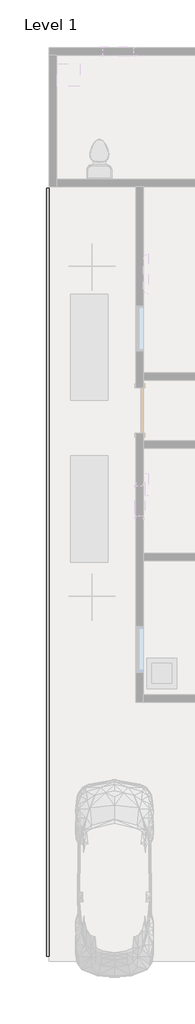
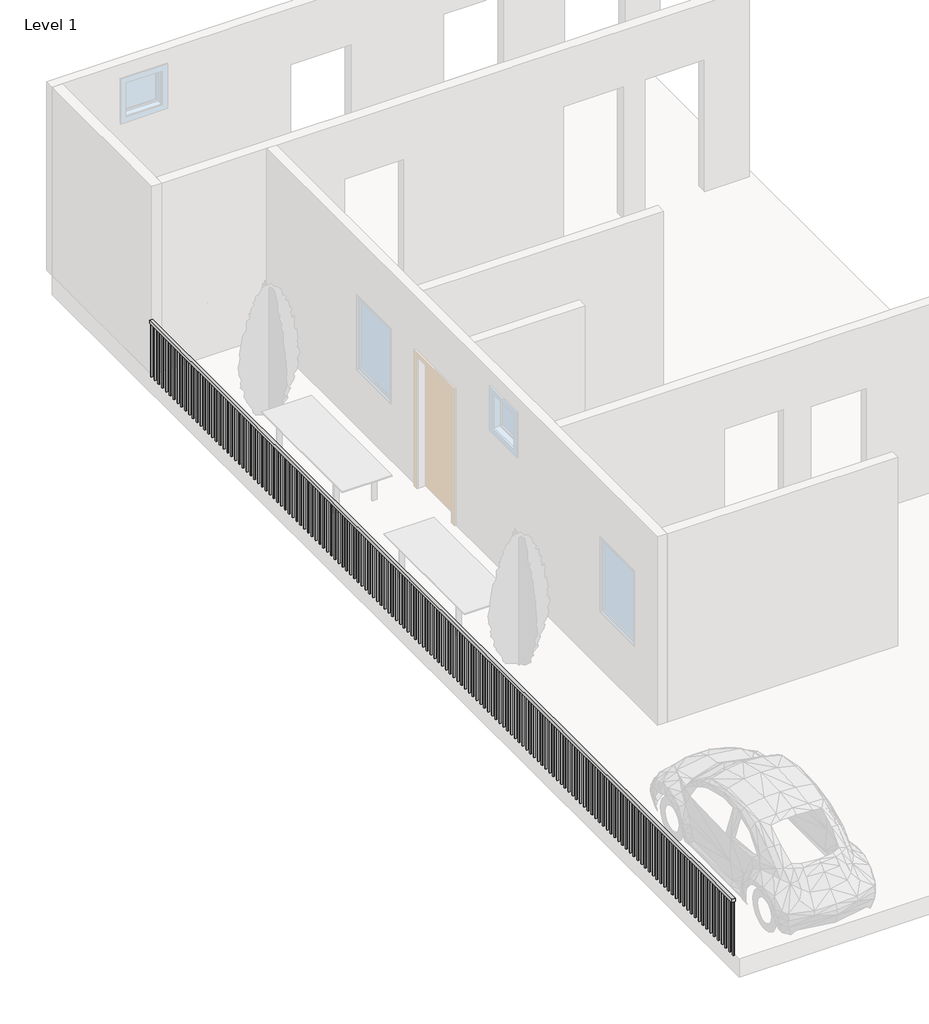
# One storey, part 3 of 4: 1 railing.
"""IFC4 building model written with IfcOpenShell, lengths in millimetres."""

from ifc_helpers import new_model, si_unit, frame, origin, origin_with_axes, place, context, project, spatial, polyline, outline, extrude, element, save

model = new_model("IFC4")

# Units and contexts
model_context = context("Model", 3, world=origin())
ifc_project = project(units=[si_unit("LENGTHUNIT", "METRE", prefix="MILLI")], contexts=[model_context])

# Site, building, storey
site = spatial("IfcSite", under=ifc_project)
building = spatial("IfcBuilding", under=site)
storey = spatial("IfcBuildingStorey", under=building, Name="Level 1", Elevation=0.0)

# Railing
placement = place(None, origin())
element("IfcRailing", 1, ObjectType="Handrail - Rectangular", at=placement, inside=storey, context=model_context, shape_type="SweptSolid", body=[
    extrude(outline(polyline([(-12085.860887, 10860.7910469), (-12035.060887, 10860.7910469), (-12035.060887, -4582.4089531), (-12085.860887, -4582.4089531), (-12085.860887, 10860.7910469)])), frame((0.0, 0.0, 863.6), z_axis=(0.0, 0.0, 1.0), x_axis=(1.0, 0.0, 0.0)), (0.0, 0.0, 1.0), 50.8),
    extrude(outline(polyline([(-12069.985887, -4471.2839531), (-12050.935887, -4471.2839531), (-12050.935887, -4490.3339531), (-12069.985887, -4490.3339531), (-12069.985887, -4471.2839531)])), origin_with_axes(), (0.0, 0.0, 1.0), 863.6),
    extrude(outline(polyline([(-12069.985887, -4369.6839531), (-12050.935887, -4369.6839531), (-12050.935887, -4388.7339531), (-12069.985887, -4388.7339531), (-12069.985887, -4369.6839531)])), origin_with_axes(), (0.0, 0.0, 1.0), 863.6),
    extrude(outline(polyline([(-12069.985887, -4268.0839531), (-12050.935887, -4268.0839531), (-12050.935887, -4287.1339531), (-12069.985887, -4287.1339531), (-12069.985887, -4268.0839531)])), origin_with_axes(), (0.0, 0.0, 1.0), 863.6),
    extrude(outline(polyline([(-12069.985887, -4166.4839531), (-12050.935887, -4166.4839531), (-12050.935887, -4185.5339531), (-12069.985887, -4185.5339531), (-12069.985887, -4166.4839531)])), origin_with_axes(), (0.0, 0.0, 1.0), 863.6),
    extrude(outline(polyline([(-12069.985887, -4064.8839531), (-12050.935887, -4064.8839531), (-12050.935887, -4083.9339531), (-12069.985887, -4083.9339531), (-12069.985887, -4064.8839531)])), origin_with_axes(), (0.0, 0.0, 1.0), 863.6),
    extrude(outline(polyline([(-12069.985887, -3963.2839531), (-12050.935887, -3963.2839531), (-12050.935887, -3982.3339531), (-12069.985887, -3982.3339531), (-12069.985887, -3963.2839531)])), origin_with_axes(), (0.0, 0.0, 1.0), 863.6),
    extrude(outline(polyline([(-12069.985887, -3861.6839531), (-12050.935887, -3861.6839531), (-12050.935887, -3880.7339531), (-12069.985887, -3880.7339531), (-12069.985887, -3861.6839531)])), origin_with_axes(), (0.0, 0.0, 1.0), 863.6),
    extrude(outline(polyline([(-12069.985887, -3760.0839531), (-12050.935887, -3760.0839531), (-12050.935887, -3779.1339531), (-12069.985887, -3779.1339531), (-12069.985887, -3760.0839531)])), origin_with_axes(), (0.0, 0.0, 1.0), 863.6),
    extrude(outline(polyline([(-12069.985887, -3658.4839531), (-12050.935887, -3658.4839531), (-12050.935887, -3677.5339531), (-12069.985887, -3677.5339531), (-12069.985887, -3658.4839531)])), origin_with_axes(), (0.0, 0.0, 1.0), 863.6),
    extrude(outline(polyline([(-12069.985887, -3556.8839531), (-12050.935887, -3556.8839531), (-12050.935887, -3575.9339531), (-12069.985887, -3575.9339531), (-12069.985887, -3556.8839531)])), origin_with_axes(), (0.0, 0.0, 1.0), 863.6),
    extrude(outline(polyline([(-12069.985887, -3455.2839531), (-12050.935887, -3455.2839531), (-12050.935887, -3474.3339531), (-12069.985887, -3474.3339531), (-12069.985887, -3455.2839531)])), origin_with_axes(), (0.0, 0.0, 1.0), 863.6),
    extrude(outline(polyline([(-12069.985887, -3353.6839531), (-12050.935887, -3353.6839531), (-12050.935887, -3372.7339531), (-12069.985887, -3372.7339531), (-12069.985887, -3353.6839531)])), origin_with_axes(), (0.0, 0.0, 1.0), 863.6),
    extrude(outline(polyline([(-12069.985887, -3252.0839531), (-12050.935887, -3252.0839531), (-12050.935887, -3271.1339531), (-12069.985887, -3271.1339531), (-12069.985887, -3252.0839531)])), origin_with_axes(), (0.0, 0.0, 1.0), 863.6),
    extrude(outline(polyline([(-12069.985887, -3150.4839531), (-12050.935887, -3150.4839531), (-12050.935887, -3169.5339531), (-12069.985887, -3169.5339531), (-12069.985887, -3150.4839531)])), origin_with_axes(), (0.0, 0.0, 1.0), 863.6),
    extrude(outline(polyline([(-12069.985887, -3048.8839531), (-12050.935887, -3048.8839531), (-12050.935887, -3067.9339531), (-12069.985887, -3067.9339531), (-12069.985887, -3048.8839531)])), origin_with_axes(), (0.0, 0.0, 1.0), 863.6),
    extrude(outline(polyline([(-12069.985887, -2947.2839531), (-12050.935887, -2947.2839531), (-12050.935887, -2966.3339531), (-12069.985887, -2966.3339531), (-12069.985887, -2947.2839531)])), origin_with_axes(), (0.0, 0.0, 1.0), 863.6),
    extrude(outline(polyline([(-12069.985887, -2845.6839531), (-12050.935887, -2845.6839531), (-12050.935887, -2864.7339531), (-12069.985887, -2864.7339531), (-12069.985887, -2845.6839531)])), origin_with_axes(), (0.0, 0.0, 1.0), 863.6),
    extrude(outline(polyline([(-12069.985887, -2744.0839531), (-12050.935887, -2744.0839531), (-12050.935887, -2763.1339531), (-12069.985887, -2763.1339531), (-12069.985887, -2744.0839531)])), origin_with_axes(), (0.0, 0.0, 1.0), 863.6),
    extrude(outline(polyline([(-12069.985887, -2642.4839531), (-12050.935887, -2642.4839531), (-12050.935887, -2661.5339531), (-12069.985887, -2661.5339531), (-12069.985887, -2642.4839531)])), origin_with_axes(), (0.0, 0.0, 1.0), 863.6),
    extrude(outline(polyline([(-12069.985887, -2540.8839531), (-12050.935887, -2540.8839531), (-12050.935887, -2559.9339531), (-12069.985887, -2559.9339531), (-12069.985887, -2540.8839531)])), origin_with_axes(), (0.0, 0.0, 1.0), 863.6),
    extrude(outline(polyline([(-12069.985887, -2439.2839531), (-12050.935887, -2439.2839531), (-12050.935887, -2458.3339531), (-12069.985887, -2458.3339531), (-12069.985887, -2439.2839531)])), origin_with_axes(), (0.0, 0.0, 1.0), 863.6),
    extrude(outline(polyline([(-12069.985887, -2337.6839531), (-12050.935887, -2337.6839531), (-12050.935887, -2356.7339531), (-12069.985887, -2356.7339531), (-12069.985887, -2337.6839531)])), origin_with_axes(), (0.0, 0.0, 1.0), 863.6),
    extrude(outline(polyline([(-12069.985887, -2236.0839531), (-12050.935887, -2236.0839531), (-12050.935887, -2255.1339531), (-12069.985887, -2255.1339531), (-12069.985887, -2236.0839531)])), origin_with_axes(), (0.0, 0.0, 1.0), 863.6),
    extrude(outline(polyline([(-12069.985887, -2134.4839531), (-12050.935887, -2134.4839531), (-12050.935887, -2153.5339531), (-12069.985887, -2153.5339531), (-12069.985887, -2134.4839531)])), origin_with_axes(), (0.0, 0.0, 1.0), 863.6),
    extrude(outline(polyline([(-12069.985887, -2032.8839531), (-12050.935887, -2032.8839531), (-12050.935887, -2051.9339531), (-12069.985887, -2051.9339531), (-12069.985887, -2032.8839531)])), origin_with_axes(), (0.0, 0.0, 1.0), 863.6),
    extrude(outline(polyline([(-12069.985887, -1931.2839531), (-12050.935887, -1931.2839531), (-12050.935887, -1950.3339531), (-12069.985887, -1950.3339531), (-12069.985887, -1931.2839531)])), origin_with_axes(), (0.0, 0.0, 1.0), 863.6),
    extrude(outline(polyline([(-12069.985887, -1829.6839531), (-12050.935887, -1829.6839531), (-12050.935887, -1848.7339531), (-12069.985887, -1848.7339531), (-12069.985887, -1829.6839531)])), origin_with_axes(), (0.0, 0.0, 1.0), 863.6),
    extrude(outline(polyline([(-12069.985887, -1728.0839531), (-12050.935887, -1728.0839531), (-12050.935887, -1747.1339531), (-12069.985887, -1747.1339531), (-12069.985887, -1728.0839531)])), origin_with_axes(), (0.0, 0.0, 1.0), 863.6),
    extrude(outline(polyline([(-12069.985887, -1626.4839531), (-12050.935887, -1626.4839531), (-12050.935887, -1645.5339531), (-12069.985887, -1645.5339531), (-12069.985887, -1626.4839531)])), origin_with_axes(), (0.0, 0.0, 1.0), 863.6),
    extrude(outline(polyline([(-12069.985887, -1524.8839531), (-12050.935887, -1524.8839531), (-12050.935887, -1543.9339531), (-12069.985887, -1543.9339531), (-12069.985887, -1524.8839531)])), origin_with_axes(), (0.0, 0.0, 1.0), 863.6),
    extrude(outline(polyline([(-12069.985887, -1423.2839531), (-12050.935887, -1423.2839531), (-12050.935887, -1442.3339531), (-12069.985887, -1442.3339531), (-12069.985887, -1423.2839531)])), origin_with_axes(), (0.0, 0.0, 1.0), 863.6),
    extrude(outline(polyline([(-12069.985887, -1321.6839531), (-12050.935887, -1321.6839531), (-12050.935887, -1340.7339531), (-12069.985887, -1340.7339531), (-12069.985887, -1321.6839531)])), origin_with_axes(), (0.0, 0.0, 1.0), 863.6),
    extrude(outline(polyline([(-12069.985887, -1220.0839531), (-12050.935887, -1220.0839531), (-12050.935887, -1239.1339531), (-12069.985887, -1239.1339531), (-12069.985887, -1220.0839531)])), origin_with_axes(), (0.0, 0.0, 1.0), 863.6),
    extrude(outline(polyline([(-12069.985887, -1118.4839531), (-12050.935887, -1118.4839531), (-12050.935887, -1137.5339531), (-12069.985887, -1137.5339531), (-12069.985887, -1118.4839531)])), origin_with_axes(), (0.0, 0.0, 1.0), 863.6),
    extrude(outline(polyline([(-12069.985887, -1016.8839531), (-12050.935887, -1016.8839531), (-12050.935887, -1035.9339531), (-12069.985887, -1035.9339531), (-12069.985887, -1016.8839531)])), origin_with_axes(), (0.0, 0.0, 1.0), 863.6),
    extrude(outline(polyline([(-12069.985887, -915.2839531), (-12050.935887, -915.2839531), (-12050.935887, -934.3339531), (-12069.985887, -934.3339531), (-12069.985887, -915.2839531)])), origin_with_axes(), (0.0, 0.0, 1.0), 863.6),
    extrude(outline(polyline([(-12069.985887, -813.6839531), (-12050.935887, -813.6839531), (-12050.935887, -832.7339531), (-12069.985887, -832.7339531), (-12069.985887, -813.6839531)])), origin_with_axes(), (0.0, 0.0, 1.0), 863.6),
    extrude(outline(polyline([(-12069.985887, -712.0839531), (-12050.935887, -712.0839531), (-12050.935887, -731.1339531), (-12069.985887, -731.1339531), (-12069.985887, -712.0839531)])), origin_with_axes(), (0.0, 0.0, 1.0), 863.6),
    extrude(outline(polyline([(-12069.985887, -610.4839531), (-12050.935887, -610.4839531), (-12050.935887, -629.5339531), (-12069.985887, -629.5339531), (-12069.985887, -610.4839531)])), origin_with_axes(), (0.0, 0.0, 1.0), 863.6),
    extrude(outline(polyline([(-12069.985887, -508.8839531), (-12050.935887, -508.8839531), (-12050.935887, -527.9339531), (-12069.985887, -527.9339531), (-12069.985887, -508.8839531)])), origin_with_axes(), (0.0, 0.0, 1.0), 863.6),
    extrude(outline(polyline([(-12069.985887, -407.2839531), (-12050.935887, -407.2839531), (-12050.935887, -426.3339531), (-12069.985887, -426.3339531), (-12069.985887, -407.2839531)])), origin_with_axes(), (0.0, 0.0, 1.0), 863.6),
    extrude(outline(polyline([(-12069.985887, -305.6839531), (-12050.935887, -305.6839531), (-12050.935887, -324.7339531), (-12069.985887, -324.7339531), (-12069.985887, -305.6839531)])), origin_with_axes(), (0.0, 0.0, 1.0), 863.6),
    extrude(outline(polyline([(-12069.985887, -204.0839531), (-12050.935887, -204.0839531), (-12050.935887, -223.1339531), (-12069.985887, -223.1339531), (-12069.985887, -204.0839531)])), origin_with_axes(), (0.0, 0.0, 1.0), 863.6),
    extrude(outline(polyline([(-12069.985887, -102.4839531), (-12050.935887, -102.4839531), (-12050.935887, -121.5339531), (-12069.985887, -121.5339531), (-12069.985887, -102.4839531)])), origin_with_axes(), (0.0, 0.0, 1.0), 863.6),
    extrude(outline(polyline([(-12069.985887, -0.8839531), (-12050.935887, -0.8839531), (-12050.935887, -19.9339531), (-12069.985887, -19.9339531), (-12069.985887, -0.8839531)])), origin_with_axes(), (0.0, 0.0, 1.0), 863.6),
    extrude(outline(polyline([(-12069.985887, 100.7160469), (-12050.935887, 100.7160469), (-12050.935887, 81.6660469), (-12069.985887, 81.6660469), (-12069.985887, 100.7160469)])), origin_with_axes(), (0.0, 0.0, 1.0), 863.6),
    extrude(outline(polyline([(-12069.985887, 202.3160469), (-12050.935887, 202.3160469), (-12050.935887, 183.2660469), (-12069.985887, 183.2660469), (-12069.985887, 202.3160469)])), origin_with_axes(), (0.0, 0.0, 1.0), 863.6),
    extrude(outline(polyline([(-12069.985887, 303.9160469), (-12050.935887, 303.9160469), (-12050.935887, 284.8660469), (-12069.985887, 284.8660469), (-12069.985887, 303.9160469)])), origin_with_axes(), (0.0, 0.0, 1.0), 863.6),
    extrude(outline(polyline([(-12069.985887, 405.5160469), (-12050.935887, 405.5160469), (-12050.935887, 386.4660469), (-12069.985887, 386.4660469), (-12069.985887, 405.5160469)])), origin_with_axes(), (0.0, 0.0, 1.0), 863.6),
    extrude(outline(polyline([(-12069.985887, 507.1160469), (-12050.935887, 507.1160469), (-12050.935887, 488.0660469), (-12069.985887, 488.0660469), (-12069.985887, 507.1160469)])), origin_with_axes(), (0.0, 0.0, 1.0), 863.6),
    extrude(outline(polyline([(-12069.985887, 608.7160469), (-12050.935887, 608.7160469), (-12050.935887, 589.6660469), (-12069.985887, 589.6660469), (-12069.985887, 608.7160469)])), origin_with_axes(), (0.0, 0.0, 1.0), 863.6),
    extrude(outline(polyline([(-12069.985887, 710.3160469), (-12050.935887, 710.3160469), (-12050.935887, 691.2660469), (-12069.985887, 691.2660469), (-12069.985887, 710.3160469)])), origin_with_axes(), (0.0, 0.0, 1.0), 863.6),
    extrude(outline(polyline([(-12069.985887, 811.9160469), (-12050.935887, 811.9160469), (-12050.935887, 792.8660469), (-12069.985887, 792.8660469), (-12069.985887, 811.9160469)])), origin_with_axes(), (0.0, 0.0, 1.0), 863.6),
    extrude(outline(polyline([(-12069.985887, 913.5160469), (-12050.935887, 913.5160469), (-12050.935887, 894.4660469), (-12069.985887, 894.4660469), (-12069.985887, 913.5160469)])), origin_with_axes(), (0.0, 0.0, 1.0), 863.6),
    extrude(outline(polyline([(-12069.985887, 1015.1160469), (-12050.935887, 1015.1160469), (-12050.935887, 996.0660469), (-12069.985887, 996.0660469), (-12069.985887, 1015.1160469)])), origin_with_axes(), (0.0, 0.0, 1.0), 863.6),
    extrude(outline(polyline([(-12069.985887, 1116.7160469), (-12050.935887, 1116.7160469), (-12050.935887, 1097.6660469), (-12069.985887, 1097.6660469), (-12069.985887, 1116.7160469)])), origin_with_axes(), (0.0, 0.0, 1.0), 863.6),
    extrude(outline(polyline([(-12069.985887, 1218.3160469), (-12050.935887, 1218.3160469), (-12050.935887, 1199.2660469), (-12069.985887, 1199.2660469), (-12069.985887, 1218.3160469)])), origin_with_axes(), (0.0, 0.0, 1.0), 863.6),
    extrude(outline(polyline([(-12069.985887, 1319.9160469), (-12050.935887, 1319.9160469), (-12050.935887, 1300.8660469), (-12069.985887, 1300.8660469), (-12069.985887, 1319.9160469)])), origin_with_axes(), (0.0, 0.0, 1.0), 863.6),
    extrude(outline(polyline([(-12069.985887, 1421.5160469), (-12050.935887, 1421.5160469), (-12050.935887, 1402.4660469), (-12069.985887, 1402.4660469), (-12069.985887, 1421.5160469)])), origin_with_axes(), (0.0, 0.0, 1.0), 863.6),
    extrude(outline(polyline([(-12069.985887, 1523.1160469), (-12050.935887, 1523.1160469), (-12050.935887, 1504.0660469), (-12069.985887, 1504.0660469), (-12069.985887, 1523.1160469)])), origin_with_axes(), (0.0, 0.0, 1.0), 863.6),
    extrude(outline(polyline([(-12069.985887, 1624.7160469), (-12050.935887, 1624.7160469), (-12050.935887, 1605.6660469), (-12069.985887, 1605.6660469), (-12069.985887, 1624.7160469)])), origin_with_axes(), (0.0, 0.0, 1.0), 863.6),
    extrude(outline(polyline([(-12069.985887, 1726.3160469), (-12050.935887, 1726.3160469), (-12050.935887, 1707.2660469), (-12069.985887, 1707.2660469), (-12069.985887, 1726.3160469)])), origin_with_axes(), (0.0, 0.0, 1.0), 863.6),
    extrude(outline(polyline([(-12069.985887, 1827.9160469), (-12050.935887, 1827.9160469), (-12050.935887, 1808.8660469), (-12069.985887, 1808.8660469), (-12069.985887, 1827.9160469)])), origin_with_axes(), (0.0, 0.0, 1.0), 863.6),
    extrude(outline(polyline([(-12069.985887, 1929.5160469), (-12050.935887, 1929.5160469), (-12050.935887, 1910.4660469), (-12069.985887, 1910.4660469), (-12069.985887, 1929.5160469)])), origin_with_axes(), (0.0, 0.0, 1.0), 863.6),
    extrude(outline(polyline([(-12069.985887, 2031.1160469), (-12050.935887, 2031.1160469), (-12050.935887, 2012.0660469), (-12069.985887, 2012.0660469), (-12069.985887, 2031.1160469)])), origin_with_axes(), (0.0, 0.0, 1.0), 863.6),
    extrude(outline(polyline([(-12069.985887, 2132.7160469), (-12050.935887, 2132.7160469), (-12050.935887, 2113.6660469), (-12069.985887, 2113.6660469), (-12069.985887, 2132.7160469)])), origin_with_axes(), (0.0, 0.0, 1.0), 863.6),
    extrude(outline(polyline([(-12069.985887, 2234.3160469), (-12050.935887, 2234.3160469), (-12050.935887, 2215.2660469), (-12069.985887, 2215.2660469), (-12069.985887, 2234.3160469)])), origin_with_axes(), (0.0, 0.0, 1.0), 863.6),
    extrude(outline(polyline([(-12069.985887, 2335.9160469), (-12050.935887, 2335.9160469), (-12050.935887, 2316.8660469), (-12069.985887, 2316.8660469), (-12069.985887, 2335.9160469)])), origin_with_axes(), (0.0, 0.0, 1.0), 863.6),
    extrude(outline(polyline([(-12069.985887, 2437.5160469), (-12050.935887, 2437.5160469), (-12050.935887, 2418.4660469), (-12069.985887, 2418.4660469), (-12069.985887, 2437.5160469)])), origin_with_axes(), (0.0, 0.0, 1.0), 863.6),
    extrude(outline(polyline([(-12069.985887, 2539.1160469), (-12050.935887, 2539.1160469), (-12050.935887, 2520.0660469), (-12069.985887, 2520.0660469), (-12069.985887, 2539.1160469)])), origin_with_axes(), (0.0, 0.0, 1.0), 863.6),
    extrude(outline(polyline([(-12069.985887, 2640.7160469), (-12050.935887, 2640.7160469), (-12050.935887, 2621.6660469), (-12069.985887, 2621.6660469), (-12069.985887, 2640.7160469)])), origin_with_axes(), (0.0, 0.0, 1.0), 863.6),
    extrude(outline(polyline([(-12069.985887, 2742.3160469), (-12050.935887, 2742.3160469), (-12050.935887, 2723.2660469), (-12069.985887, 2723.2660469), (-12069.985887, 2742.3160469)])), origin_with_axes(), (0.0, 0.0, 1.0), 863.6),
    extrude(outline(polyline([(-12069.985887, 2843.9160469), (-12050.935887, 2843.9160469), (-12050.935887, 2824.8660469), (-12069.985887, 2824.8660469), (-12069.985887, 2843.9160469)])), origin_with_axes(), (0.0, 0.0, 1.0), 863.6),
    extrude(outline(polyline([(-12069.985887, 2945.5160469), (-12050.935887, 2945.5160469), (-12050.935887, 2926.4660469), (-12069.985887, 2926.4660469), (-12069.985887, 2945.5160469)])), origin_with_axes(), (0.0, 0.0, 1.0), 863.6),
    extrude(outline(polyline([(-12069.985887, 3047.1160469), (-12050.935887, 3047.1160469), (-12050.935887, 3028.0660469), (-12069.985887, 3028.0660469), (-12069.985887, 3047.1160469)])), origin_with_axes(), (0.0, 0.0, 1.0), 863.6),
    extrude(outline(polyline([(-12069.985887, 3148.7160469), (-12050.935887, 3148.7160469), (-12050.935887, 3129.6660469), (-12069.985887, 3129.6660469), (-12069.985887, 3148.7160469)])), origin_with_axes(), (0.0, 0.0, 1.0), 863.6),
    extrude(outline(polyline([(-12069.985887, 3250.3160469), (-12050.935887, 3250.3160469), (-12050.935887, 3231.2660469), (-12069.985887, 3231.2660469), (-12069.985887, 3250.3160469)])), origin_with_axes(), (0.0, 0.0, 1.0), 863.6),
    extrude(outline(polyline([(-12069.985887, 3351.9160469), (-12050.935887, 3351.9160469), (-12050.935887, 3332.8660469), (-12069.985887, 3332.8660469), (-12069.985887, 3351.9160469)])), origin_with_axes(), (0.0, 0.0, 1.0), 863.6),
    extrude(outline(polyline([(-12069.985887, 3453.5160469), (-12050.935887, 3453.5160469), (-12050.935887, 3434.4660469), (-12069.985887, 3434.4660469), (-12069.985887, 3453.5160469)])), origin_with_axes(), (0.0, 0.0, 1.0), 863.6),
    extrude(outline(polyline([(-12069.985887, 3555.1160469), (-12050.935887, 3555.1160469), (-12050.935887, 3536.0660469), (-12069.985887, 3536.0660469), (-12069.985887, 3555.1160469)])), origin_with_axes(), (0.0, 0.0, 1.0), 863.6),
    extrude(outline(polyline([(-12069.985887, 3656.7160469), (-12050.935887, 3656.7160469), (-12050.935887, 3637.6660469), (-12069.985887, 3637.6660469), (-12069.985887, 3656.7160469)])), origin_with_axes(), (0.0, 0.0, 1.0), 863.6),
    extrude(outline(polyline([(-12069.985887, 3758.3160469), (-12050.935887, 3758.3160469), (-12050.935887, 3739.2660469), (-12069.985887, 3739.2660469), (-12069.985887, 3758.3160469)])), origin_with_axes(), (0.0, 0.0, 1.0), 863.6),
    extrude(outline(polyline([(-12069.985887, 3859.9160469), (-12050.935887, 3859.9160469), (-12050.935887, 3840.8660469), (-12069.985887, 3840.8660469), (-12069.985887, 3859.9160469)])), origin_with_axes(), (0.0, 0.0, 1.0), 863.6),
    extrude(outline(polyline([(-12069.985887, 3961.5160469), (-12050.935887, 3961.5160469), (-12050.935887, 3942.4660469), (-12069.985887, 3942.4660469), (-12069.985887, 3961.5160469)])), origin_with_axes(), (0.0, 0.0, 1.0), 863.6),
    extrude(outline(polyline([(-12069.985887, 4063.1160469), (-12050.935887, 4063.1160469), (-12050.935887, 4044.0660469), (-12069.985887, 4044.0660469), (-12069.985887, 4063.1160469)])), origin_with_axes(), (0.0, 0.0, 1.0), 863.6),
    extrude(outline(polyline([(-12069.985887, 4164.7160469), (-12050.935887, 4164.7160469), (-12050.935887, 4145.6660469), (-12069.985887, 4145.6660469), (-12069.985887, 4164.7160469)])), origin_with_axes(), (0.0, 0.0, 1.0), 863.6),
    extrude(outline(polyline([(-12069.985887, 4266.3160469), (-12050.935887, 4266.3160469), (-12050.935887, 4247.2660469), (-12069.985887, 4247.2660469), (-12069.985887, 4266.3160469)])), origin_with_axes(), (0.0, 0.0, 1.0), 863.6),
    extrude(outline(polyline([(-12069.985887, 4367.9160469), (-12050.935887, 4367.9160469), (-12050.935887, 4348.8660469), (-12069.985887, 4348.8660469), (-12069.985887, 4367.9160469)])), origin_with_axes(), (0.0, 0.0, 1.0), 863.6),
    extrude(outline(polyline([(-12069.985887, 4469.5160469), (-12050.935887, 4469.5160469), (-12050.935887, 4450.4660469), (-12069.985887, 4450.4660469), (-12069.985887, 4469.5160469)])), origin_with_axes(), (0.0, 0.0, 1.0), 863.6),
    extrude(outline(polyline([(-12069.985887, 4571.1160469), (-12050.935887, 4571.1160469), (-12050.935887, 4552.0660469), (-12069.985887, 4552.0660469), (-12069.985887, 4571.1160469)])), origin_with_axes(), (0.0, 0.0, 1.0), 863.6),
    extrude(outline(polyline([(-12069.985887, 4672.7160469), (-12050.935887, 4672.7160469), (-12050.935887, 4653.6660469), (-12069.985887, 4653.6660469), (-12069.985887, 4672.7160469)])), origin_with_axes(), (0.0, 0.0, 1.0), 863.6),
    extrude(outline(polyline([(-12069.985887, 4774.3160469), (-12050.935887, 4774.3160469), (-12050.935887, 4755.2660469), (-12069.985887, 4755.2660469), (-12069.985887, 4774.3160469)])), origin_with_axes(), (0.0, 0.0, 1.0), 863.6),
    extrude(outline(polyline([(-12069.985887, 4875.9160469), (-12050.935887, 4875.9160469), (-12050.935887, 4856.8660469), (-12069.985887, 4856.8660469), (-12069.985887, 4875.9160469)])), origin_with_axes(), (0.0, 0.0, 1.0), 863.6),
    extrude(outline(polyline([(-12069.985887, 4977.5160469), (-12050.935887, 4977.5160469), (-12050.935887, 4958.4660469), (-12069.985887, 4958.4660469), (-12069.985887, 4977.5160469)])), origin_with_axes(), (0.0, 0.0, 1.0), 863.6),
    extrude(outline(polyline([(-12069.985887, 5079.1160469), (-12050.935887, 5079.1160469), (-12050.935887, 5060.0660469), (-12069.985887, 5060.0660469), (-12069.985887, 5079.1160469)])), origin_with_axes(), (0.0, 0.0, 1.0), 863.6),
    extrude(outline(polyline([(-12069.985887, 5180.7160469), (-12050.935887, 5180.7160469), (-12050.935887, 5161.6660469), (-12069.985887, 5161.6660469), (-12069.985887, 5180.7160469)])), origin_with_axes(), (0.0, 0.0, 1.0), 863.6),
    extrude(outline(polyline([(-12069.985887, 5282.3160469), (-12050.935887, 5282.3160469), (-12050.935887, 5263.2660469), (-12069.985887, 5263.2660469), (-12069.985887, 5282.3160469)])), origin_with_axes(), (0.0, 0.0, 1.0), 863.6),
    extrude(outline(polyline([(-12069.985887, 5383.9160469), (-12050.935887, 5383.9160469), (-12050.935887, 5364.8660469), (-12069.985887, 5364.8660469), (-12069.985887, 5383.9160469)])), origin_with_axes(), (0.0, 0.0, 1.0), 863.6),
    extrude(outline(polyline([(-12069.985887, 5485.5160469), (-12050.935887, 5485.5160469), (-12050.935887, 5466.4660469), (-12069.985887, 5466.4660469), (-12069.985887, 5485.5160469)])), origin_with_axes(), (0.0, 0.0, 1.0), 863.6),
    extrude(outline(polyline([(-12069.985887, 5587.1160469), (-12050.935887, 5587.1160469), (-12050.935887, 5568.0660469), (-12069.985887, 5568.0660469), (-12069.985887, 5587.1160469)])), origin_with_axes(), (0.0, 0.0, 1.0), 863.6),
    extrude(outline(polyline([(-12069.985887, 5688.7160469), (-12050.935887, 5688.7160469), (-12050.935887, 5669.6660469), (-12069.985887, 5669.6660469), (-12069.985887, 5688.7160469)])), origin_with_axes(), (0.0, 0.0, 1.0), 863.6),
    extrude(outline(polyline([(-12069.985887, 5790.3160469), (-12050.935887, 5790.3160469), (-12050.935887, 5771.2660469), (-12069.985887, 5771.2660469), (-12069.985887, 5790.3160469)])), origin_with_axes(), (0.0, 0.0, 1.0), 863.6),
    extrude(outline(polyline([(-12069.985887, 5891.9160469), (-12050.935887, 5891.9160469), (-12050.935887, 5872.8660469), (-12069.985887, 5872.8660469), (-12069.985887, 5891.9160469)])), origin_with_axes(), (0.0, 0.0, 1.0), 863.6),
    extrude(outline(polyline([(-12069.985887, 5993.5160469), (-12050.935887, 5993.5160469), (-12050.935887, 5974.4660469), (-12069.985887, 5974.4660469), (-12069.985887, 5993.5160469)])), origin_with_axes(), (0.0, 0.0, 1.0), 863.6),
    extrude(outline(polyline([(-12069.985887, 6095.1160469), (-12050.935887, 6095.1160469), (-12050.935887, 6076.0660469), (-12069.985887, 6076.0660469), (-12069.985887, 6095.1160469)])), origin_with_axes(), (0.0, 0.0, 1.0), 863.6),
    extrude(outline(polyline([(-12069.985887, 6196.7160469), (-12050.935887, 6196.7160469), (-12050.935887, 6177.6660469), (-12069.985887, 6177.6660469), (-12069.985887, 6196.7160469)])), origin_with_axes(), (0.0, 0.0, 1.0), 863.6),
    extrude(outline(polyline([(-12069.985887, 6298.3160469), (-12050.935887, 6298.3160469), (-12050.935887, 6279.2660469), (-12069.985887, 6279.2660469), (-12069.985887, 6298.3160469)])), origin_with_axes(), (0.0, 0.0, 1.0), 863.6),
    extrude(outline(polyline([(-12069.985887, 6399.9160469), (-12050.935887, 6399.9160469), (-12050.935887, 6380.8660469), (-12069.985887, 6380.8660469), (-12069.985887, 6399.9160469)])), origin_with_axes(), (0.0, 0.0, 1.0), 863.6),
    extrude(outline(polyline([(-12069.985887, 6501.5160469), (-12050.935887, 6501.5160469), (-12050.935887, 6482.4660469), (-12069.985887, 6482.4660469), (-12069.985887, 6501.5160469)])), origin_with_axes(), (0.0, 0.0, 1.0), 863.6),
    extrude(outline(polyline([(-12069.985887, 6603.1160469), (-12050.935887, 6603.1160469), (-12050.935887, 6584.0660469), (-12069.985887, 6584.0660469), (-12069.985887, 6603.1160469)])), origin_with_axes(), (0.0, 0.0, 1.0), 863.6),
    extrude(outline(polyline([(-12069.985887, 6704.7160469), (-12050.935887, 6704.7160469), (-12050.935887, 6685.6660469), (-12069.985887, 6685.6660469), (-12069.985887, 6704.7160469)])), origin_with_axes(), (0.0, 0.0, 1.0), 863.6),
    extrude(outline(polyline([(-12069.985887, 6806.3160469), (-12050.935887, 6806.3160469), (-12050.935887, 6787.2660469), (-12069.985887, 6787.2660469), (-12069.985887, 6806.3160469)])), origin_with_axes(), (0.0, 0.0, 1.0), 863.6),
    extrude(outline(polyline([(-12069.985887, 6907.9160469), (-12050.935887, 6907.9160469), (-12050.935887, 6888.8660469), (-12069.985887, 6888.8660469), (-12069.985887, 6907.9160469)])), origin_with_axes(), (0.0, 0.0, 1.0), 863.6),
    extrude(outline(polyline([(-12069.985887, 7009.5160469), (-12050.935887, 7009.5160469), (-12050.935887, 6990.4660469), (-12069.985887, 6990.4660469), (-12069.985887, 7009.5160469)])), origin_with_axes(), (0.0, 0.0, 1.0), 863.6),
    extrude(outline(polyline([(-12069.985887, 7111.1160469), (-12050.935887, 7111.1160469), (-12050.935887, 7092.0660469), (-12069.985887, 7092.0660469), (-12069.985887, 7111.1160469)])), origin_with_axes(), (0.0, 0.0, 1.0), 863.6),
    extrude(outline(polyline([(-12069.985887, 7212.7160469), (-12050.935887, 7212.7160469), (-12050.935887, 7193.6660469), (-12069.985887, 7193.6660469), (-12069.985887, 7212.7160469)])), origin_with_axes(), (0.0, 0.0, 1.0), 863.6),
    extrude(outline(polyline([(-12069.985887, 7314.3160469), (-12050.935887, 7314.3160469), (-12050.935887, 7295.2660469), (-12069.985887, 7295.2660469), (-12069.985887, 7314.3160469)])), origin_with_axes(), (0.0, 0.0, 1.0), 863.6),
    extrude(outline(polyline([(-12069.985887, 7415.9160469), (-12050.935887, 7415.9160469), (-12050.935887, 7396.8660469), (-12069.985887, 7396.8660469), (-12069.985887, 7415.9160469)])), origin_with_axes(), (0.0, 0.0, 1.0), 863.6),
    extrude(outline(polyline([(-12069.985887, 7517.5160469), (-12050.935887, 7517.5160469), (-12050.935887, 7498.4660469), (-12069.985887, 7498.4660469), (-12069.985887, 7517.5160469)])), origin_with_axes(), (0.0, 0.0, 1.0), 863.6),
    extrude(outline(polyline([(-12069.985887, 7619.1160469), (-12050.935887, 7619.1160469), (-12050.935887, 7600.0660469), (-12069.985887, 7600.0660469), (-12069.985887, 7619.1160469)])), origin_with_axes(), (0.0, 0.0, 1.0), 863.6),
    extrude(outline(polyline([(-12069.985887, 7720.7160469), (-12050.935887, 7720.7160469), (-12050.935887, 7701.6660469), (-12069.985887, 7701.6660469), (-12069.985887, 7720.7160469)])), origin_with_axes(), (0.0, 0.0, 1.0), 863.6),
    extrude(outline(polyline([(-12069.985887, 7822.3160469), (-12050.935887, 7822.3160469), (-12050.935887, 7803.2660469), (-12069.985887, 7803.2660469), (-12069.985887, 7822.3160469)])), origin_with_axes(), (0.0, 0.0, 1.0), 863.6),
    extrude(outline(polyline([(-12069.985887, 7923.9160469), (-12050.935887, 7923.9160469), (-12050.935887, 7904.8660469), (-12069.985887, 7904.8660469), (-12069.985887, 7923.9160469)])), origin_with_axes(), (0.0, 0.0, 1.0), 863.6),
    extrude(outline(polyline([(-12069.985887, 8025.5160469), (-12050.935887, 8025.5160469), (-12050.935887, 8006.4660469), (-12069.985887, 8006.4660469), (-12069.985887, 8025.5160469)])), origin_with_axes(), (0.0, 0.0, 1.0), 863.6),
    extrude(outline(polyline([(-12069.985887, 8127.1160469), (-12050.935887, 8127.1160469), (-12050.935887, 8108.0660469), (-12069.985887, 8108.0660469), (-12069.985887, 8127.1160469)])), origin_with_axes(), (0.0, 0.0, 1.0), 863.6),
    extrude(outline(polyline([(-12069.985887, 8228.7160469), (-12050.935887, 8228.7160469), (-12050.935887, 8209.6660469), (-12069.985887, 8209.6660469), (-12069.985887, 8228.7160469)])), origin_with_axes(), (0.0, 0.0, 1.0), 863.6),
    extrude(outline(polyline([(-12069.985887, 8330.3160469), (-12050.935887, 8330.3160469), (-12050.935887, 8311.2660469), (-12069.985887, 8311.2660469), (-12069.985887, 8330.3160469)])), origin_with_axes(), (0.0, 0.0, 1.0), 863.6),
    extrude(outline(polyline([(-12069.985887, 8431.9160469), (-12050.935887, 8431.9160469), (-12050.935887, 8412.8660469), (-12069.985887, 8412.8660469), (-12069.985887, 8431.9160469)])), origin_with_axes(), (0.0, 0.0, 1.0), 863.6),
    extrude(outline(polyline([(-12069.985887, 8533.5160469), (-12050.935887, 8533.5160469), (-12050.935887, 8514.4660469), (-12069.985887, 8514.4660469), (-12069.985887, 8533.5160469)])), origin_with_axes(), (0.0, 0.0, 1.0), 863.6),
    extrude(outline(polyline([(-12069.985887, 8635.1160469), (-12050.935887, 8635.1160469), (-12050.935887, 8616.0660469), (-12069.985887, 8616.0660469), (-12069.985887, 8635.1160469)])), origin_with_axes(), (0.0, 0.0, 1.0), 863.6),
    extrude(outline(polyline([(-12069.985887, 8736.7160469), (-12050.935887, 8736.7160469), (-12050.935887, 8717.6660469), (-12069.985887, 8717.6660469), (-12069.985887, 8736.7160469)])), origin_with_axes(), (0.0, 0.0, 1.0), 863.6),
    extrude(outline(polyline([(-12069.985887, 8838.3160469), (-12050.935887, 8838.3160469), (-12050.935887, 8819.2660469), (-12069.985887, 8819.2660469), (-12069.985887, 8838.3160469)])), origin_with_axes(), (0.0, 0.0, 1.0), 863.6),
    extrude(outline(polyline([(-12069.985887, 8939.9160469), (-12050.935887, 8939.9160469), (-12050.935887, 8920.8660469), (-12069.985887, 8920.8660469), (-12069.985887, 8939.9160469)])), origin_with_axes(), (0.0, 0.0, 1.0), 863.6),
    extrude(outline(polyline([(-12069.985887, 9041.5160469), (-12050.935887, 9041.5160469), (-12050.935887, 9022.4660469), (-12069.985887, 9022.4660469), (-12069.985887, 9041.5160469)])), origin_with_axes(), (0.0, 0.0, 1.0), 863.6),
    extrude(outline(polyline([(-12069.985887, 9143.1160469), (-12050.935887, 9143.1160469), (-12050.935887, 9124.0660469), (-12069.985887, 9124.0660469), (-12069.985887, 9143.1160469)])), origin_with_axes(), (0.0, 0.0, 1.0), 863.6),
    extrude(outline(polyline([(-12069.985887, 9244.7160469), (-12050.935887, 9244.7160469), (-12050.935887, 9225.6660469), (-12069.985887, 9225.6660469), (-12069.985887, 9244.7160469)])), origin_with_axes(), (0.0, 0.0, 1.0), 863.6),
    extrude(outline(polyline([(-12069.985887, 9346.3160469), (-12050.935887, 9346.3160469), (-12050.935887, 9327.2660469), (-12069.985887, 9327.2660469), (-12069.985887, 9346.3160469)])), origin_with_axes(), (0.0, 0.0, 1.0), 863.6),
    extrude(outline(polyline([(-12069.985887, 9447.9160469), (-12050.935887, 9447.9160469), (-12050.935887, 9428.8660469), (-12069.985887, 9428.8660469), (-12069.985887, 9447.9160469)])), origin_with_axes(), (0.0, 0.0, 1.0), 863.6),
    extrude(outline(polyline([(-12069.985887, 9549.5160469), (-12050.935887, 9549.5160469), (-12050.935887, 9530.4660469), (-12069.985887, 9530.4660469), (-12069.985887, 9549.5160469)])), origin_with_axes(), (0.0, 0.0, 1.0), 863.6),
    extrude(outline(polyline([(-12069.985887, 9651.1160469), (-12050.935887, 9651.1160469), (-12050.935887, 9632.0660469), (-12069.985887, 9632.0660469), (-12069.985887, 9651.1160469)])), origin_with_axes(), (0.0, 0.0, 1.0), 863.6),
    extrude(outline(polyline([(-12069.985887, 9752.7160469), (-12050.935887, 9752.7160469), (-12050.935887, 9733.6660469), (-12069.985887, 9733.6660469), (-12069.985887, 9752.7160469)])), origin_with_axes(), (0.0, 0.0, 1.0), 863.6),
    extrude(outline(polyline([(-12069.985887, 9854.3160469), (-12050.935887, 9854.3160469), (-12050.935887, 9835.2660469), (-12069.985887, 9835.2660469), (-12069.985887, 9854.3160469)])), origin_with_axes(), (0.0, 0.0, 1.0), 863.6),
    extrude(outline(polyline([(-12069.985887, 9955.9160469), (-12050.935887, 9955.9160469), (-12050.935887, 9936.8660469), (-12069.985887, 9936.8660469), (-12069.985887, 9955.9160469)])), origin_with_axes(), (0.0, 0.0, 1.0), 863.6),
    extrude(outline(polyline([(-12069.985887, 10057.5160469), (-12050.935887, 10057.5160469), (-12050.935887, 10038.4660469), (-12069.985887, 10038.4660469), (-12069.985887, 10057.5160469)])), origin_with_axes(), (0.0, 0.0, 1.0), 863.6),
    extrude(outline(polyline([(-12069.985887, 10159.1160469), (-12050.935887, 10159.1160469), (-12050.935887, 10140.0660469), (-12069.985887, 10140.0660469), (-12069.985887, 10159.1160469)])), origin_with_axes(), (0.0, 0.0, 1.0), 863.6),
    extrude(outline(polyline([(-12069.985887, 10260.7160469), (-12050.935887, 10260.7160469), (-12050.935887, 10241.6660469), (-12069.985887, 10241.6660469), (-12069.985887, 10260.7160469)])), origin_with_axes(), (0.0, 0.0, 1.0), 863.6),
    extrude(outline(polyline([(-12069.985887, 10362.3160469), (-12050.935887, 10362.3160469), (-12050.935887, 10343.2660469), (-12069.985887, 10343.2660469), (-12069.985887, 10362.3160469)])), origin_with_axes(), (0.0, 0.0, 1.0), 863.6),
    extrude(outline(polyline([(-12069.985887, 10463.9160469), (-12050.935887, 10463.9160469), (-12050.935887, 10444.8660469), (-12069.985887, 10444.8660469), (-12069.985887, 10463.9160469)])), origin_with_axes(), (0.0, 0.0, 1.0), 863.6),
    extrude(outline(polyline([(-12069.985887, 10565.5160469), (-12050.935887, 10565.5160469), (-12050.935887, 10546.4660469), (-12069.985887, 10546.4660469), (-12069.985887, 10565.5160469)])), origin_with_axes(), (0.0, 0.0, 1.0), 863.6),
    extrude(outline(polyline([(-12069.985887, 10667.1160469), (-12050.935887, 10667.1160469), (-12050.935887, 10648.0660469), (-12069.985887, 10648.0660469), (-12069.985887, 10667.1160469)])), origin_with_axes(), (0.0, 0.0, 1.0), 863.6),
    extrude(outline(polyline([(-12069.985887, 10768.7160469), (-12050.935887, 10768.7160469), (-12050.935887, 10749.6660469), (-12069.985887, 10749.6660469), (-12069.985887, 10768.7160469)])), origin_with_axes(), (0.0, 0.0, 1.0), 863.6),
    extrude(outline(polyline([(-12069.985887, -4563.3589531), (-12050.935887, -4563.3589531), (-12050.935887, -4582.4089531), (-12069.985887, -4582.4089531), (-12069.985887, -4563.3589531)])), origin_with_axes(), (0.0, 0.0, 1.0), 863.6),
    extrude(outline(polyline([(-12069.985887, 10860.7910469), (-12050.935887, 10860.7910469), (-12050.935887, 10841.7410469), (-12069.985887, 10841.7410469), (-12069.985887, 10860.7910469)])), origin_with_axes(), (0.0, 0.0, 1.0), 863.6),
])

save(model, "model.ifc")

# Revit data of these elements
# Type "Handrail - Rectangular"
#   Assembly Code = "C2010400"
#   built-in parameter 1008612 = 0.0416667 (stored number, unit not read)
#   built-in parameter 1008611 = 0.0416667 (stored number, unit not read)
#   built-in parameter 1008609 = 0.333333 (stored number, unit not read)
#   built-in parameter 1008604 = 0.166667 (stored number, unit not read)
#   built-in parameter 1008603 = 0.166667 (stored number, unit not read)
#   Railing Height = 3' - 0"
#   built-in parameter 1008630 = 2
#   built-in parameter 1008610 = 2
#   built-in parameter 1008618 = Baluster - Square : 3/4"
# Element 1 (IfcRailing, "Handrail - Rectangular")
#   Phase Created = New Construction
